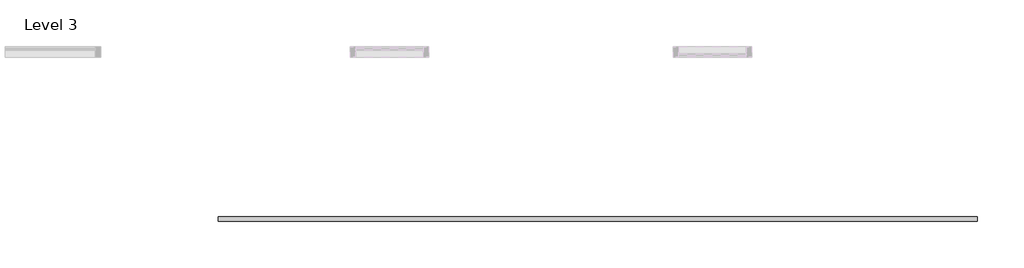
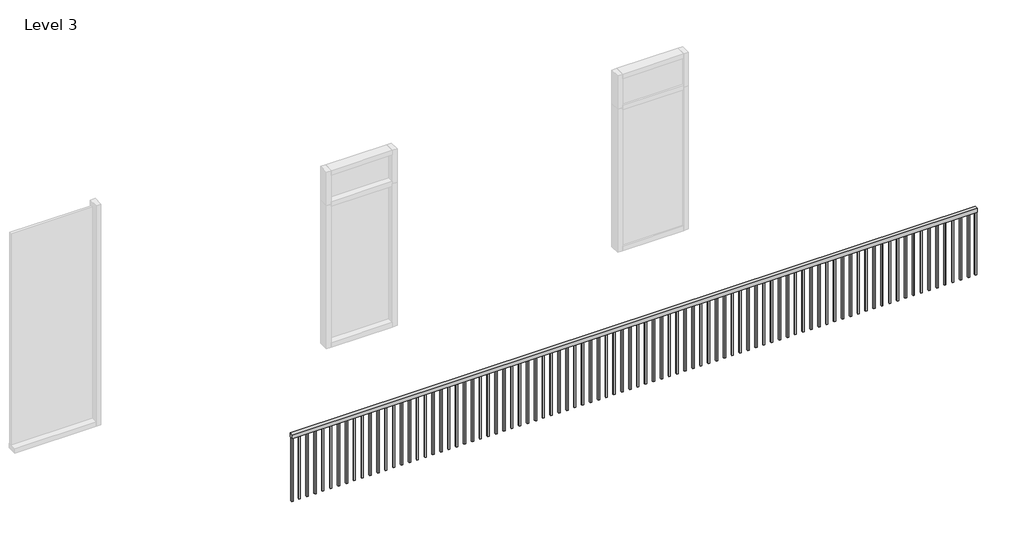
# One storey, part 2 of 2: 1 railing.
"""IFC4 building model written with IfcOpenShell, lengths in millimetres."""

from ifc_helpers import new_model, si_unit, frame, origin, place, context, project, spatial, polyline, outline, extrude, element, save

model = new_model("IFC4")

# Units and contexts
model_context = context("Model", 3, world=origin())
ifc_project = project(units=[si_unit("LENGTHUNIT", "METRE", prefix="MILLI")], contexts=[model_context])

# Site, building, storey
site = spatial("IfcSite", under=ifc_project)
building = spatial("IfcBuilding", under=site)
storey = spatial("IfcBuildingStorey", under=building, Name="Level 3", Elevation=4318.0)

# Railing
placement = place(None, origin())
element("IfcRailing", 1, ObjectType="Handrail - Rectangular", at=placement, inside=storey, context=model_context, shape_type="SweptSolid", body=[
    extrude(outline(polyline([(6694.2940915, -4895.9585517), (6694.2940915, -4946.7585517), (-2144.9059085, -4946.7585517), (-2144.9059085, -4895.9585517), (6694.2940915, -4895.9585517)])), frame((0.0, 0.0, 5181.6), z_axis=(0.0, 0.0, 1.0), x_axis=(1.0, 0.0, 0.0)), (0.0, 0.0, 1.0), 50.8),
    extrude(outline(polyline([(-2033.7809085, -4911.8335517), (-2033.7809085, -4930.8835517), (-2052.8309085, -4930.8835517), (-2052.8309085, -4911.8335517), (-2033.7809085, -4911.8335517)])), frame((0.0, 0.0, 4318.0), z_axis=(0.0, 0.0, 1.0), x_axis=(1.0, 0.0, 0.0)), (0.0, 0.0, 1.0), 863.6),
    extrude(outline(polyline([(-1932.1809085, -4911.8335517), (-1932.1809085, -4930.8835517), (-1951.2309085, -4930.8835517), (-1951.2309085, -4911.8335517), (-1932.1809085, -4911.8335517)])), frame((0.0, 0.0, 4318.0), z_axis=(0.0, 0.0, 1.0), x_axis=(1.0, 0.0, 0.0)), (0.0, 0.0, 1.0), 863.6),
    extrude(outline(polyline([(-1830.5809085, -4911.8335517), (-1830.5809085, -4930.8835517), (-1849.6309085, -4930.8835517), (-1849.6309085, -4911.8335517), (-1830.5809085, -4911.8335517)])), frame((0.0, 0.0, 4318.0), z_axis=(0.0, 0.0, 1.0), x_axis=(1.0, 0.0, 0.0)), (0.0, 0.0, 1.0), 863.6),
    extrude(outline(polyline([(-1728.9809085, -4911.8335517), (-1728.9809085, -4930.8835517), (-1748.0309085, -4930.8835517), (-1748.0309085, -4911.8335517), (-1728.9809085, -4911.8335517)])), frame((0.0, 0.0, 4318.0), z_axis=(0.0, 0.0, 1.0), x_axis=(1.0, 0.0, 0.0)), (0.0, 0.0, 1.0), 863.6),
    extrude(outline(polyline([(-1627.3809085, -4911.8335517), (-1627.3809085, -4930.8835517), (-1646.4309085, -4930.8835517), (-1646.4309085, -4911.8335517), (-1627.3809085, -4911.8335517)])), frame((0.0, 0.0, 4318.0), z_axis=(0.0, 0.0, 1.0), x_axis=(1.0, 0.0, 0.0)), (0.0, 0.0, 1.0), 863.6),
    extrude(outline(polyline([(-1525.7809085, -4911.8335517), (-1525.7809085, -4930.8835517), (-1544.8309085, -4930.8835517), (-1544.8309085, -4911.8335517), (-1525.7809085, -4911.8335517)])), frame((0.0, 0.0, 4318.0), z_axis=(0.0, 0.0, 1.0), x_axis=(1.0, 0.0, 0.0)), (0.0, 0.0, 1.0), 863.6),
    extrude(outline(polyline([(-1424.1809085, -4911.8335517), (-1424.1809085, -4930.8835517), (-1443.2309085, -4930.8835517), (-1443.2309085, -4911.8335517), (-1424.1809085, -4911.8335517)])), frame((0.0, 0.0, 4318.0), z_axis=(0.0, 0.0, 1.0), x_axis=(1.0, 0.0, 0.0)), (0.0, 0.0, 1.0), 863.6),
    extrude(outline(polyline([(-1322.5809085, -4911.8335517), (-1322.5809085, -4930.8835517), (-1341.6309085, -4930.8835517), (-1341.6309085, -4911.8335517), (-1322.5809085, -4911.8335517)])), frame((0.0, 0.0, 4318.0), z_axis=(0.0, 0.0, 1.0), x_axis=(1.0, 0.0, 0.0)), (0.0, 0.0, 1.0), 863.6),
    extrude(outline(polyline([(-1220.9809085, -4911.8335517), (-1220.9809085, -4930.8835517), (-1240.0309085, -4930.8835517), (-1240.0309085, -4911.8335517), (-1220.9809085, -4911.8335517)])), frame((0.0, 0.0, 4318.0), z_axis=(0.0, 0.0, 1.0), x_axis=(1.0, 0.0, 0.0)), (0.0, 0.0, 1.0), 863.6),
    extrude(outline(polyline([(-1119.3809085, -4911.8335517), (-1119.3809085, -4930.8835517), (-1138.4309085, -4930.8835517), (-1138.4309085, -4911.8335517), (-1119.3809085, -4911.8335517)])), frame((0.0, 0.0, 4318.0), z_axis=(0.0, 0.0, 1.0), x_axis=(1.0, 0.0, 0.0)), (0.0, 0.0, 1.0), 863.6),
    extrude(outline(polyline([(-1017.7809085, -4911.8335517), (-1017.7809085, -4930.8835517), (-1036.8309085, -4930.8835517), (-1036.8309085, -4911.8335517), (-1017.7809085, -4911.8335517)])), frame((0.0, 0.0, 4318.0), z_axis=(0.0, 0.0, 1.0), x_axis=(1.0, 0.0, 0.0)), (0.0, 0.0, 1.0), 863.6),
    extrude(outline(polyline([(-916.1809085, -4911.8335517), (-916.1809085, -4930.8835517), (-935.2309085, -4930.8835517), (-935.2309085, -4911.8335517), (-916.1809085, -4911.8335517)])), frame((0.0, 0.0, 4318.0), z_axis=(0.0, 0.0, 1.0), x_axis=(1.0, 0.0, 0.0)), (0.0, 0.0, 1.0), 863.6),
    extrude(outline(polyline([(-814.5809085, -4911.8335517), (-814.5809085, -4930.8835517), (-833.6309085, -4930.8835517), (-833.6309085, -4911.8335517), (-814.5809085, -4911.8335517)])), frame((0.0, 0.0, 4318.0), z_axis=(0.0, 0.0, 1.0), x_axis=(1.0, 0.0, 0.0)), (0.0, 0.0, 1.0), 863.6),
    extrude(outline(polyline([(-712.9809085, -4911.8335517), (-712.9809085, -4930.8835517), (-732.0309085, -4930.8835517), (-732.0309085, -4911.8335517), (-712.9809085, -4911.8335517)])), frame((0.0, 0.0, 4318.0), z_axis=(0.0, 0.0, 1.0), x_axis=(1.0, 0.0, 0.0)), (0.0, 0.0, 1.0), 863.6),
    extrude(outline(polyline([(-611.3809085, -4911.8335517), (-611.3809085, -4930.8835517), (-630.4309085, -4930.8835517), (-630.4309085, -4911.8335517), (-611.3809085, -4911.8335517)])), frame((0.0, 0.0, 4318.0), z_axis=(0.0, 0.0, 1.0), x_axis=(1.0, 0.0, 0.0)), (0.0, 0.0, 1.0), 863.6),
    extrude(outline(polyline([(-509.7809085, -4911.8335517), (-509.7809085, -4930.8835517), (-528.8309085, -4930.8835517), (-528.8309085, -4911.8335517), (-509.7809085, -4911.8335517)])), frame((0.0, 0.0, 4318.0), z_axis=(0.0, 0.0, 1.0), x_axis=(1.0, 0.0, 0.0)), (0.0, 0.0, 1.0), 863.6),
    extrude(outline(polyline([(-408.1809085, -4911.8335517), (-408.1809085, -4930.8835517), (-427.2309085, -4930.8835517), (-427.2309085, -4911.8335517), (-408.1809085, -4911.8335517)])), frame((0.0, 0.0, 4318.0), z_axis=(0.0, 0.0, 1.0), x_axis=(1.0, 0.0, 0.0)), (0.0, 0.0, 1.0), 863.6),
    extrude(outline(polyline([(-306.5809085, -4911.8335517), (-306.5809085, -4930.8835517), (-325.6309085, -4930.8835517), (-325.6309085, -4911.8335517), (-306.5809085, -4911.8335517)])), frame((0.0, 0.0, 4318.0), z_axis=(0.0, 0.0, 1.0), x_axis=(1.0, 0.0, 0.0)), (0.0, 0.0, 1.0), 863.6),
    extrude(outline(polyline([(-204.9809085, -4911.8335517), (-204.9809085, -4930.8835517), (-224.0309085, -4930.8835517), (-224.0309085, -4911.8335517), (-204.9809085, -4911.8335517)])), frame((0.0, 0.0, 4318.0), z_axis=(0.0, 0.0, 1.0), x_axis=(1.0, 0.0, 0.0)), (0.0, 0.0, 1.0), 863.6),
    extrude(outline(polyline([(-103.3809085, -4911.8335517), (-103.3809085, -4930.8835517), (-122.4309085, -4930.8835517), (-122.4309085, -4911.8335517), (-103.3809085, -4911.8335517)])), frame((0.0, 0.0, 4318.0), z_axis=(0.0, 0.0, 1.0), x_axis=(1.0, 0.0, 0.0)), (0.0, 0.0, 1.0), 863.6),
    extrude(outline(polyline([(-1.7809085, -4911.8335517), (-1.7809085, -4930.8835517), (-20.8309085, -4930.8835517), (-20.8309085, -4911.8335517), (-1.7809085, -4911.8335517)])), frame((0.0, 0.0, 4318.0), z_axis=(0.0, 0.0, 1.0), x_axis=(1.0, 0.0, 0.0)), (0.0, 0.0, 1.0), 863.6),
    extrude(outline(polyline([(99.8190915, -4911.8335517), (99.8190915, -4930.8835517), (80.7690915, -4930.8835517), (80.7690915, -4911.8335517), (99.8190915, -4911.8335517)])), frame((0.0, 0.0, 4318.0), z_axis=(0.0, 0.0, 1.0), x_axis=(1.0, 0.0, 0.0)), (0.0, 0.0, 1.0), 863.6),
    extrude(outline(polyline([(201.4190915, -4911.8335517), (201.4190915, -4930.8835517), (182.3690915, -4930.8835517), (182.3690915, -4911.8335517), (201.4190915, -4911.8335517)])), frame((0.0, 0.0, 4318.0), z_axis=(0.0, 0.0, 1.0), x_axis=(1.0, 0.0, 0.0)), (0.0, 0.0, 1.0), 863.6),
    extrude(outline(polyline([(303.0190915, -4911.8335517), (303.0190915, -4930.8835517), (283.9690915, -4930.8835517), (283.9690915, -4911.8335517), (303.0190915, -4911.8335517)])), frame((0.0, 0.0, 4318.0), z_axis=(0.0, 0.0, 1.0), x_axis=(1.0, 0.0, 0.0)), (0.0, 0.0, 1.0), 863.6),
    extrude(outline(polyline([(404.6190915, -4911.8335517), (404.6190915, -4930.8835517), (385.5690915, -4930.8835517), (385.5690915, -4911.8335517), (404.6190915, -4911.8335517)])), frame((0.0, 0.0, 4318.0), z_axis=(0.0, 0.0, 1.0), x_axis=(1.0, 0.0, 0.0)), (0.0, 0.0, 1.0), 863.6),
    extrude(outline(polyline([(506.2190915, -4911.8335517), (506.2190915, -4930.8835517), (487.1690915, -4930.8835517), (487.1690915, -4911.8335517), (506.2190915, -4911.8335517)])), frame((0.0, 0.0, 4318.0), z_axis=(0.0, 0.0, 1.0), x_axis=(1.0, 0.0, 0.0)), (0.0, 0.0, 1.0), 863.6),
    extrude(outline(polyline([(607.8190915, -4911.8335517), (607.8190915, -4930.8835517), (588.7690915, -4930.8835517), (588.7690915, -4911.8335517), (607.8190915, -4911.8335517)])), frame((0.0, 0.0, 4318.0), z_axis=(0.0, 0.0, 1.0), x_axis=(1.0, 0.0, 0.0)), (0.0, 0.0, 1.0), 863.6),
    extrude(outline(polyline([(709.4190915, -4911.8335517), (709.4190915, -4930.8835517), (690.3690915, -4930.8835517), (690.3690915, -4911.8335517), (709.4190915, -4911.8335517)])), frame((0.0, 0.0, 4318.0), z_axis=(0.0, 0.0, 1.0), x_axis=(1.0, 0.0, 0.0)), (0.0, 0.0, 1.0), 863.6),
    extrude(outline(polyline([(811.0190915, -4911.8335517), (811.0190915, -4930.8835517), (791.9690915, -4930.8835517), (791.9690915, -4911.8335517), (811.0190915, -4911.8335517)])), frame((0.0, 0.0, 4318.0), z_axis=(0.0, 0.0, 1.0), x_axis=(1.0, 0.0, 0.0)), (0.0, 0.0, 1.0), 863.6),
    extrude(outline(polyline([(912.6190915, -4911.8335517), (912.6190915, -4930.8835517), (893.5690915, -4930.8835517), (893.5690915, -4911.8335517), (912.6190915, -4911.8335517)])), frame((0.0, 0.0, 4318.0), z_axis=(0.0, 0.0, 1.0), x_axis=(1.0, 0.0, 0.0)), (0.0, 0.0, 1.0), 863.6),
    extrude(outline(polyline([(1014.2190915, -4911.8335517), (1014.2190915, -4930.8835517), (995.1690915, -4930.8835517), (995.1690915, -4911.8335517), (1014.2190915, -4911.8335517)])), frame((0.0, 0.0, 4318.0), z_axis=(0.0, 0.0, 1.0), x_axis=(1.0, 0.0, 0.0)), (0.0, 0.0, 1.0), 863.6),
    extrude(outline(polyline([(1115.8190915, -4911.8335517), (1115.8190915, -4930.8835517), (1096.7690915, -4930.8835517), (1096.7690915, -4911.8335517), (1115.8190915, -4911.8335517)])), frame((0.0, 0.0, 4318.0), z_axis=(0.0, 0.0, 1.0), x_axis=(1.0, 0.0, 0.0)), (0.0, 0.0, 1.0), 863.6),
    extrude(outline(polyline([(1217.4190915, -4911.8335517), (1217.4190915, -4930.8835517), (1198.3690915, -4930.8835517), (1198.3690915, -4911.8335517), (1217.4190915, -4911.8335517)])), frame((0.0, 0.0, 4318.0), z_axis=(0.0, 0.0, 1.0), x_axis=(1.0, 0.0, 0.0)), (0.0, 0.0, 1.0), 863.6),
    extrude(outline(polyline([(1319.0190915, -4911.8335517), (1319.0190915, -4930.8835517), (1299.9690915, -4930.8835517), (1299.9690915, -4911.8335517), (1319.0190915, -4911.8335517)])), frame((0.0, 0.0, 4318.0), z_axis=(0.0, 0.0, 1.0), x_axis=(1.0, 0.0, 0.0)), (0.0, 0.0, 1.0), 863.6),
    extrude(outline(polyline([(1420.6190915, -4911.8335517), (1420.6190915, -4930.8835517), (1401.5690915, -4930.8835517), (1401.5690915, -4911.8335517), (1420.6190915, -4911.8335517)])), frame((0.0, 0.0, 4318.0), z_axis=(0.0, 0.0, 1.0), x_axis=(1.0, 0.0, 0.0)), (0.0, 0.0, 1.0), 863.6),
    extrude(outline(polyline([(1522.2190915, -4911.8335517), (1522.2190915, -4930.8835517), (1503.1690915, -4930.8835517), (1503.1690915, -4911.8335517), (1522.2190915, -4911.8335517)])), frame((0.0, 0.0, 4318.0), z_axis=(0.0, 0.0, 1.0), x_axis=(1.0, 0.0, 0.0)), (0.0, 0.0, 1.0), 863.6),
    extrude(outline(polyline([(1623.8190915, -4911.8335517), (1623.8190915, -4930.8835517), (1604.7690915, -4930.8835517), (1604.7690915, -4911.8335517), (1623.8190915, -4911.8335517)])), frame((0.0, 0.0, 4318.0), z_axis=(0.0, 0.0, 1.0), x_axis=(1.0, 0.0, 0.0)), (0.0, 0.0, 1.0), 863.6),
    extrude(outline(polyline([(1725.4190915, -4911.8335517), (1725.4190915, -4930.8835517), (1706.3690915, -4930.8835517), (1706.3690915, -4911.8335517), (1725.4190915, -4911.8335517)])), frame((0.0, 0.0, 4318.0), z_axis=(0.0, 0.0, 1.0), x_axis=(1.0, 0.0, 0.0)), (0.0, 0.0, 1.0), 863.6),
    extrude(outline(polyline([(1827.0190915, -4911.8335517), (1827.0190915, -4930.8835517), (1807.9690915, -4930.8835517), (1807.9690915, -4911.8335517), (1827.0190915, -4911.8335517)])), frame((0.0, 0.0, 4318.0), z_axis=(0.0, 0.0, 1.0), x_axis=(1.0, 0.0, 0.0)), (0.0, 0.0, 1.0), 863.6),
    extrude(outline(polyline([(1928.6190915, -4911.8335517), (1928.6190915, -4930.8835517), (1909.5690915, -4930.8835517), (1909.5690915, -4911.8335517), (1928.6190915, -4911.8335517)])), frame((0.0, 0.0, 4318.0), z_axis=(0.0, 0.0, 1.0), x_axis=(1.0, 0.0, 0.0)), (0.0, 0.0, 1.0), 863.6),
    extrude(outline(polyline([(2030.2190915, -4911.8335517), (2030.2190915, -4930.8835517), (2011.1690915, -4930.8835517), (2011.1690915, -4911.8335517), (2030.2190915, -4911.8335517)])), frame((0.0, 0.0, 4318.0), z_axis=(0.0, 0.0, 1.0), x_axis=(1.0, 0.0, 0.0)), (0.0, 0.0, 1.0), 863.6),
    extrude(outline(polyline([(2131.8190915, -4911.8335517), (2131.8190915, -4930.8835517), (2112.7690915, -4930.8835517), (2112.7690915, -4911.8335517), (2131.8190915, -4911.8335517)])), frame((0.0, 0.0, 4318.0), z_axis=(0.0, 0.0, 1.0), x_axis=(1.0, 0.0, 0.0)), (0.0, 0.0, 1.0), 863.6),
    extrude(outline(polyline([(2233.4190915, -4911.8335517), (2233.4190915, -4930.8835517), (2214.3690915, -4930.8835517), (2214.3690915, -4911.8335517), (2233.4190915, -4911.8335517)])), frame((0.0, 0.0, 4318.0), z_axis=(0.0, 0.0, 1.0), x_axis=(1.0, 0.0, 0.0)), (0.0, 0.0, 1.0), 863.6),
    extrude(outline(polyline([(2335.0190915, -4911.8335517), (2335.0190915, -4930.8835517), (2315.9690915, -4930.8835517), (2315.9690915, -4911.8335517), (2335.0190915, -4911.8335517)])), frame((0.0, 0.0, 4318.0), z_axis=(0.0, 0.0, 1.0), x_axis=(1.0, 0.0, 0.0)), (0.0, 0.0, 1.0), 863.6),
    extrude(outline(polyline([(2436.6190915, -4911.8335517), (2436.6190915, -4930.8835517), (2417.5690915, -4930.8835517), (2417.5690915, -4911.8335517), (2436.6190915, -4911.8335517)])), frame((0.0, 0.0, 4318.0), z_axis=(0.0, 0.0, 1.0), x_axis=(1.0, 0.0, 0.0)), (0.0, 0.0, 1.0), 863.6),
    extrude(outline(polyline([(2538.2190915, -4911.8335517), (2538.2190915, -4930.8835517), (2519.1690915, -4930.8835517), (2519.1690915, -4911.8335517), (2538.2190915, -4911.8335517)])), frame((0.0, 0.0, 4318.0), z_axis=(0.0, 0.0, 1.0), x_axis=(1.0, 0.0, 0.0)), (0.0, 0.0, 1.0), 863.6),
    extrude(outline(polyline([(2639.8190915, -4911.8335517), (2639.8190915, -4930.8835517), (2620.7690915, -4930.8835517), (2620.7690915, -4911.8335517), (2639.8190915, -4911.8335517)])), frame((0.0, 0.0, 4318.0), z_axis=(0.0, 0.0, 1.0), x_axis=(1.0, 0.0, 0.0)), (0.0, 0.0, 1.0), 863.6),
    extrude(outline(polyline([(2741.4190915, -4911.8335517), (2741.4190915, -4930.8835517), (2722.3690915, -4930.8835517), (2722.3690915, -4911.8335517), (2741.4190915, -4911.8335517)])), frame((0.0, 0.0, 4318.0), z_axis=(0.0, 0.0, 1.0), x_axis=(1.0, 0.0, 0.0)), (0.0, 0.0, 1.0), 863.6),
    extrude(outline(polyline([(2843.0190915, -4911.8335517), (2843.0190915, -4930.8835517), (2823.9690915, -4930.8835517), (2823.9690915, -4911.8335517), (2843.0190915, -4911.8335517)])), frame((0.0, 0.0, 4318.0), z_axis=(0.0, 0.0, 1.0), x_axis=(1.0, 0.0, 0.0)), (0.0, 0.0, 1.0), 863.6),
    extrude(outline(polyline([(2944.6190915, -4911.8335517), (2944.6190915, -4930.8835517), (2925.5690915, -4930.8835517), (2925.5690915, -4911.8335517), (2944.6190915, -4911.8335517)])), frame((0.0, 0.0, 4318.0), z_axis=(0.0, 0.0, 1.0), x_axis=(1.0, 0.0, 0.0)), (0.0, 0.0, 1.0), 863.6),
    extrude(outline(polyline([(3046.2190915, -4911.8335517), (3046.2190915, -4930.8835517), (3027.1690915, -4930.8835517), (3027.1690915, -4911.8335517), (3046.2190915, -4911.8335517)])), frame((0.0, 0.0, 4318.0), z_axis=(0.0, 0.0, 1.0), x_axis=(1.0, 0.0, 0.0)), (0.0, 0.0, 1.0), 863.6),
    extrude(outline(polyline([(3147.8190915, -4911.8335517), (3147.8190915, -4930.8835517), (3128.7690915, -4930.8835517), (3128.7690915, -4911.8335517), (3147.8190915, -4911.8335517)])), frame((0.0, 0.0, 4318.0), z_axis=(0.0, 0.0, 1.0), x_axis=(1.0, 0.0, 0.0)), (0.0, 0.0, 1.0), 863.6),
    extrude(outline(polyline([(3249.4190915, -4911.8335517), (3249.4190915, -4930.8835517), (3230.3690915, -4930.8835517), (3230.3690915, -4911.8335517), (3249.4190915, -4911.8335517)])), frame((0.0, 0.0, 4318.0), z_axis=(0.0, 0.0, 1.0), x_axis=(1.0, 0.0, 0.0)), (0.0, 0.0, 1.0), 863.6),
    extrude(outline(polyline([(3351.0190915, -4911.8335517), (3351.0190915, -4930.8835517), (3331.9690915, -4930.8835517), (3331.9690915, -4911.8335517), (3351.0190915, -4911.8335517)])), frame((0.0, 0.0, 4318.0), z_axis=(0.0, 0.0, 1.0), x_axis=(1.0, 0.0, 0.0)), (0.0, 0.0, 1.0), 863.6),
    extrude(outline(polyline([(3452.6190915, -4911.8335517), (3452.6190915, -4930.8835517), (3433.5690915, -4930.8835517), (3433.5690915, -4911.8335517), (3452.6190915, -4911.8335517)])), frame((0.0, 0.0, 4318.0), z_axis=(0.0, 0.0, 1.0), x_axis=(1.0, 0.0, 0.0)), (0.0, 0.0, 1.0), 863.6),
    extrude(outline(polyline([(3554.2190915, -4911.8335517), (3554.2190915, -4930.8835517), (3535.1690915, -4930.8835517), (3535.1690915, -4911.8335517), (3554.2190915, -4911.8335517)])), frame((0.0, 0.0, 4318.0), z_axis=(0.0, 0.0, 1.0), x_axis=(1.0, 0.0, 0.0)), (0.0, 0.0, 1.0), 863.6),
    extrude(outline(polyline([(3655.8190915, -4911.8335517), (3655.8190915, -4930.8835517), (3636.7690915, -4930.8835517), (3636.7690915, -4911.8335517), (3655.8190915, -4911.8335517)])), frame((0.0, 0.0, 4318.0), z_axis=(0.0, 0.0, 1.0), x_axis=(1.0, 0.0, 0.0)), (0.0, 0.0, 1.0), 863.6),
    extrude(outline(polyline([(3757.4190915, -4911.8335517), (3757.4190915, -4930.8835517), (3738.3690915, -4930.8835517), (3738.3690915, -4911.8335517), (3757.4190915, -4911.8335517)])), frame((0.0, 0.0, 4318.0), z_axis=(0.0, 0.0, 1.0), x_axis=(1.0, 0.0, 0.0)), (0.0, 0.0, 1.0), 863.6),
    extrude(outline(polyline([(3859.0190915, -4911.8335517), (3859.0190915, -4930.8835517), (3839.9690915, -4930.8835517), (3839.9690915, -4911.8335517), (3859.0190915, -4911.8335517)])), frame((0.0, 0.0, 4318.0), z_axis=(0.0, 0.0, 1.0), x_axis=(1.0, 0.0, 0.0)), (0.0, 0.0, 1.0), 863.6),
    extrude(outline(polyline([(3960.6190915, -4911.8335517), (3960.6190915, -4930.8835517), (3941.5690915, -4930.8835517), (3941.5690915, -4911.8335517), (3960.6190915, -4911.8335517)])), frame((0.0, 0.0, 4318.0), z_axis=(0.0, 0.0, 1.0), x_axis=(1.0, 0.0, 0.0)), (0.0, 0.0, 1.0), 863.6),
    extrude(outline(polyline([(4062.2190915, -4911.8335517), (4062.2190915, -4930.8835517), (4043.1690915, -4930.8835517), (4043.1690915, -4911.8335517), (4062.2190915, -4911.8335517)])), frame((0.0, 0.0, 4318.0), z_axis=(0.0, 0.0, 1.0), x_axis=(1.0, 0.0, 0.0)), (0.0, 0.0, 1.0), 863.6),
    extrude(outline(polyline([(4163.8190915, -4911.8335517), (4163.8190915, -4930.8835517), (4144.7690915, -4930.8835517), (4144.7690915, -4911.8335517), (4163.8190915, -4911.8335517)])), frame((0.0, 0.0, 4318.0), z_axis=(0.0, 0.0, 1.0), x_axis=(1.0, 0.0, 0.0)), (0.0, 0.0, 1.0), 863.6),
    extrude(outline(polyline([(4265.4190915, -4911.8335517), (4265.4190915, -4930.8835517), (4246.3690915, -4930.8835517), (4246.3690915, -4911.8335517), (4265.4190915, -4911.8335517)])), frame((0.0, 0.0, 4318.0), z_axis=(0.0, 0.0, 1.0), x_axis=(1.0, 0.0, 0.0)), (0.0, 0.0, 1.0), 863.6),
    extrude(outline(polyline([(4367.0190915, -4911.8335517), (4367.0190915, -4930.8835517), (4347.9690915, -4930.8835517), (4347.9690915, -4911.8335517), (4367.0190915, -4911.8335517)])), frame((0.0, 0.0, 4318.0), z_axis=(0.0, 0.0, 1.0), x_axis=(1.0, 0.0, 0.0)), (0.0, 0.0, 1.0), 863.6),
    extrude(outline(polyline([(4468.6190915, -4911.8335517), (4468.6190915, -4930.8835517), (4449.5690915, -4930.8835517), (4449.5690915, -4911.8335517), (4468.6190915, -4911.8335517)])), frame((0.0, 0.0, 4318.0), z_axis=(0.0, 0.0, 1.0), x_axis=(1.0, 0.0, 0.0)), (0.0, 0.0, 1.0), 863.6),
    extrude(outline(polyline([(4570.2190915, -4911.8335517), (4570.2190915, -4930.8835517), (4551.1690915, -4930.8835517), (4551.1690915, -4911.8335517), (4570.2190915, -4911.8335517)])), frame((0.0, 0.0, 4318.0), z_axis=(0.0, 0.0, 1.0), x_axis=(1.0, 0.0, 0.0)), (0.0, 0.0, 1.0), 863.6),
    extrude(outline(polyline([(4671.8190915, -4911.8335517), (4671.8190915, -4930.8835517), (4652.7690915, -4930.8835517), (4652.7690915, -4911.8335517), (4671.8190915, -4911.8335517)])), frame((0.0, 0.0, 4318.0), z_axis=(0.0, 0.0, 1.0), x_axis=(1.0, 0.0, 0.0)), (0.0, 0.0, 1.0), 863.6),
    extrude(outline(polyline([(4773.4190915, -4911.8335517), (4773.4190915, -4930.8835517), (4754.3690915, -4930.8835517), (4754.3690915, -4911.8335517), (4773.4190915, -4911.8335517)])), frame((0.0, 0.0, 4318.0), z_axis=(0.0, 0.0, 1.0), x_axis=(1.0, 0.0, 0.0)), (0.0, 0.0, 1.0), 863.6),
    extrude(outline(polyline([(4875.0190915, -4911.8335517), (4875.0190915, -4930.8835517), (4855.9690915, -4930.8835517), (4855.9690915, -4911.8335517), (4875.0190915, -4911.8335517)])), frame((0.0, 0.0, 4318.0), z_axis=(0.0, 0.0, 1.0), x_axis=(1.0, 0.0, 0.0)), (0.0, 0.0, 1.0), 863.6),
    extrude(outline(polyline([(4976.6190915, -4911.8335517), (4976.6190915, -4930.8835517), (4957.5690915, -4930.8835517), (4957.5690915, -4911.8335517), (4976.6190915, -4911.8335517)])), frame((0.0, 0.0, 4318.0), z_axis=(0.0, 0.0, 1.0), x_axis=(1.0, 0.0, 0.0)), (0.0, 0.0, 1.0), 863.6),
    extrude(outline(polyline([(5078.2190915, -4911.8335517), (5078.2190915, -4930.8835517), (5059.1690915, -4930.8835517), (5059.1690915, -4911.8335517), (5078.2190915, -4911.8335517)])), frame((0.0, 0.0, 4318.0), z_axis=(0.0, 0.0, 1.0), x_axis=(1.0, 0.0, 0.0)), (0.0, 0.0, 1.0), 863.6),
    extrude(outline(polyline([(5179.8190915, -4911.8335517), (5179.8190915, -4930.8835517), (5160.7690915, -4930.8835517), (5160.7690915, -4911.8335517), (5179.8190915, -4911.8335517)])), frame((0.0, 0.0, 4318.0), z_axis=(0.0, 0.0, 1.0), x_axis=(1.0, 0.0, 0.0)), (0.0, 0.0, 1.0), 863.6),
    extrude(outline(polyline([(5281.4190915, -4911.8335517), (5281.4190915, -4930.8835517), (5262.3690915, -4930.8835517), (5262.3690915, -4911.8335517), (5281.4190915, -4911.8335517)])), frame((0.0, 0.0, 4318.0), z_axis=(0.0, 0.0, 1.0), x_axis=(1.0, 0.0, 0.0)), (0.0, 0.0, 1.0), 863.6),
    extrude(outline(polyline([(5383.0190915, -4911.8335517), (5383.0190915, -4930.8835517), (5363.9690915, -4930.8835517), (5363.9690915, -4911.8335517), (5383.0190915, -4911.8335517)])), frame((0.0, 0.0, 4318.0), z_axis=(0.0, 0.0, 1.0), x_axis=(1.0, 0.0, 0.0)), (0.0, 0.0, 1.0), 863.6),
    extrude(outline(polyline([(5484.6190915, -4911.8335517), (5484.6190915, -4930.8835517), (5465.5690915, -4930.8835517), (5465.5690915, -4911.8335517), (5484.6190915, -4911.8335517)])), frame((0.0, 0.0, 4318.0), z_axis=(0.0, 0.0, 1.0), x_axis=(1.0, 0.0, 0.0)), (0.0, 0.0, 1.0), 863.6),
    extrude(outline(polyline([(5586.2190915, -4911.8335517), (5586.2190915, -4930.8835517), (5567.1690915, -4930.8835517), (5567.1690915, -4911.8335517), (5586.2190915, -4911.8335517)])), frame((0.0, 0.0, 4318.0), z_axis=(0.0, 0.0, 1.0), x_axis=(1.0, 0.0, 0.0)), (0.0, 0.0, 1.0), 863.6),
    extrude(outline(polyline([(5687.8190915, -4911.8335517), (5687.8190915, -4930.8835517), (5668.7690915, -4930.8835517), (5668.7690915, -4911.8335517), (5687.8190915, -4911.8335517)])), frame((0.0, 0.0, 4318.0), z_axis=(0.0, 0.0, 1.0), x_axis=(1.0, 0.0, 0.0)), (0.0, 0.0, 1.0), 863.6),
    extrude(outline(polyline([(5789.4190915, -4911.8335517), (5789.4190915, -4930.8835517), (5770.3690915, -4930.8835517), (5770.3690915, -4911.8335517), (5789.4190915, -4911.8335517)])), frame((0.0, 0.0, 4318.0), z_axis=(0.0, 0.0, 1.0), x_axis=(1.0, 0.0, 0.0)), (0.0, 0.0, 1.0), 863.6),
    extrude(outline(polyline([(5891.0190915, -4911.8335517), (5891.0190915, -4930.8835517), (5871.9690915, -4930.8835517), (5871.9690915, -4911.8335517), (5891.0190915, -4911.8335517)])), frame((0.0, 0.0, 4318.0), z_axis=(0.0, 0.0, 1.0), x_axis=(1.0, 0.0, 0.0)), (0.0, 0.0, 1.0), 863.6),
    extrude(outline(polyline([(5992.6190915, -4911.8335517), (5992.6190915, -4930.8835517), (5973.5690915, -4930.8835517), (5973.5690915, -4911.8335517), (5992.6190915, -4911.8335517)])), frame((0.0, 0.0, 4318.0), z_axis=(0.0, 0.0, 1.0), x_axis=(1.0, 0.0, 0.0)), (0.0, 0.0, 1.0), 863.6),
    extrude(outline(polyline([(6094.2190915, -4911.8335517), (6094.2190915, -4930.8835517), (6075.1690915, -4930.8835517), (6075.1690915, -4911.8335517), (6094.2190915, -4911.8335517)])), frame((0.0, 0.0, 4318.0), z_axis=(0.0, 0.0, 1.0), x_axis=(1.0, 0.0, 0.0)), (0.0, 0.0, 1.0), 863.6),
    extrude(outline(polyline([(6195.8190915, -4911.8335517), (6195.8190915, -4930.8835517), (6176.7690915, -4930.8835517), (6176.7690915, -4911.8335517), (6195.8190915, -4911.8335517)])), frame((0.0, 0.0, 4318.0), z_axis=(0.0, 0.0, 1.0), x_axis=(1.0, 0.0, 0.0)), (0.0, 0.0, 1.0), 863.6),
    extrude(outline(polyline([(6297.4190915, -4911.8335517), (6297.4190915, -4930.8835517), (6278.3690915, -4930.8835517), (6278.3690915, -4911.8335517), (6297.4190915, -4911.8335517)])), frame((0.0, 0.0, 4318.0), z_axis=(0.0, 0.0, 1.0), x_axis=(1.0, 0.0, 0.0)), (0.0, 0.0, 1.0), 863.6),
    extrude(outline(polyline([(6399.0190915, -4911.8335517), (6399.0190915, -4930.8835517), (6379.9690915, -4930.8835517), (6379.9690915, -4911.8335517), (6399.0190915, -4911.8335517)])), frame((0.0, 0.0, 4318.0), z_axis=(0.0, 0.0, 1.0), x_axis=(1.0, 0.0, 0.0)), (0.0, 0.0, 1.0), 863.6),
    extrude(outline(polyline([(6500.6190915, -4911.8335517), (6500.6190915, -4930.8835517), (6481.5690915, -4930.8835517), (6481.5690915, -4911.8335517), (6500.6190915, -4911.8335517)])), frame((0.0, 0.0, 4318.0), z_axis=(0.0, 0.0, 1.0), x_axis=(1.0, 0.0, 0.0)), (0.0, 0.0, 1.0), 863.6),
    extrude(outline(polyline([(6602.2190915, -4911.8335517), (6602.2190915, -4930.8835517), (6583.1690915, -4930.8835517), (6583.1690915, -4911.8335517), (6602.2190915, -4911.8335517)])), frame((0.0, 0.0, 4318.0), z_axis=(0.0, 0.0, 1.0), x_axis=(1.0, 0.0, 0.0)), (0.0, 0.0, 1.0), 863.6),
    extrude(outline(polyline([(-2125.8559085, -4911.8335517), (-2125.8559085, -4930.8835517), (-2144.9059085, -4930.8835517), (-2144.9059085, -4911.8335517), (-2125.8559085, -4911.8335517)])), frame((0.0, 0.0, 4318.0), z_axis=(0.0, 0.0, 1.0), x_axis=(1.0, 0.0, 0.0)), (0.0, 0.0, 1.0), 863.6),
    extrude(outline(polyline([(6694.2940915, -4911.8335517), (6694.2940915, -4930.8835517), (6675.2440915, -4930.8835517), (6675.2440915, -4911.8335517), (6694.2940915, -4911.8335517)])), frame((0.0, 0.0, 4318.0), z_axis=(0.0, 0.0, 1.0), x_axis=(1.0, 0.0, 0.0)), (0.0, 0.0, 1.0), 863.6),
])

save(model, "model.ifc")

# Revit data of these elements
# Type "Handrail - Rectangular"
#   Assembly Code = "C2010400"
#   built-in parameter 1008612 = 0.0416667 (stored number, unit not read)
#   built-in parameter 1008611 = 0.0416667 (stored number, unit not read)
#   built-in parameter 1008609 = 0.333333 (stored number, unit not read)
#   built-in parameter 1008604 = 0.166667 (stored number, unit not read)
#   built-in parameter 1008603 = 0.166667 (stored number, unit not read)
#   Railing Height = 3' - 0"
#   built-in parameter 1008630 = 2
#   built-in parameter 1008610 = 2
#   built-in parameter 1008618 = Baluster - Square : 3/4"
# Element 1 (IfcRailing, "Handrail - Rectangular")
#   Phase Created = New Construction
#   Materials on its faces: "railing"
# Materials
#   "railing": class "Generic", colour RGB 120 120 120, transparency 0, Cost = 0
